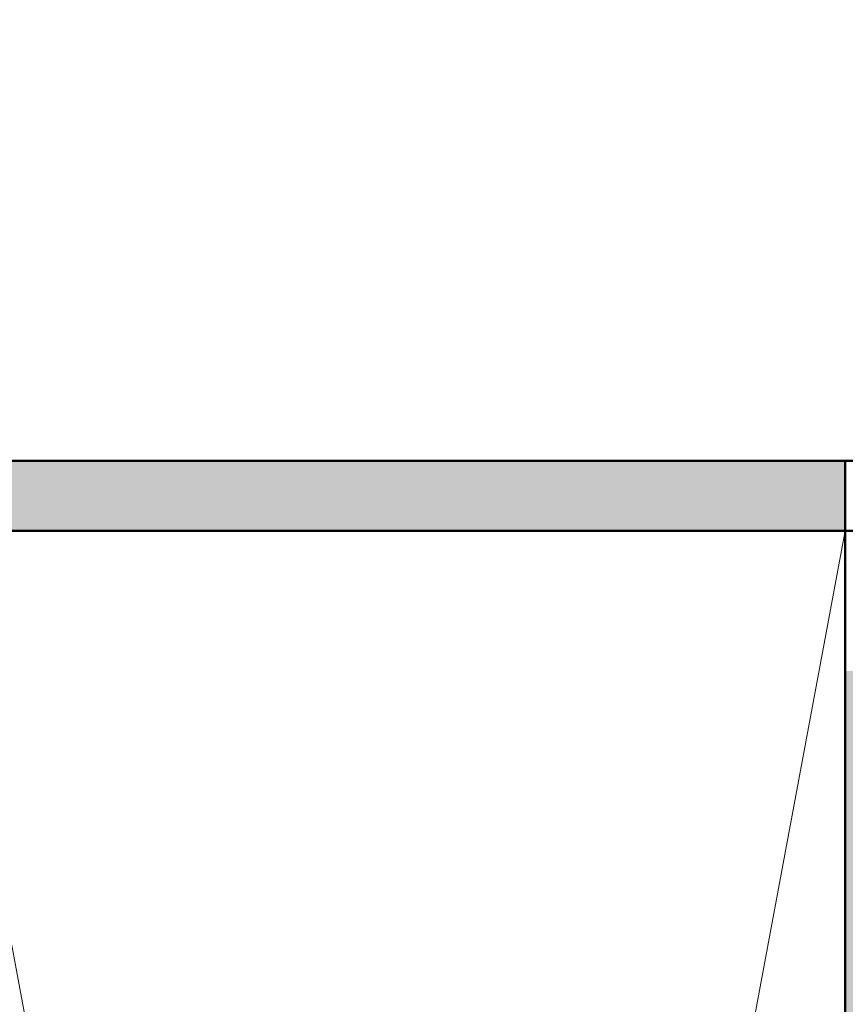
# Model space of a CAD drawing. Units: inches. Extents: x -7 to 1228, y -146 to 1091.
# Tile 28 of 88: x 563 to 634, y 446 to 531. Entities that reach past the tile are written whole.
import ezdxf

# ---------------------------------------------------------------- set-up
doc = ezdxf.new("R2010")
doc.units = ezdxf.units.IN
for name, color, linetype, lineweight in [('A-FLOR-VOID', 7, 'Continuous', 18), ('A-WALL', 7, 'Continuous', 50), ('A-WALL-PATT', 251, 'Continuous', 13)]:
    doc.layers.add(name, color=color, linetype=linetype, lineweight=lineweight)

msp = doc.modelspace()

# ---------------------------------------------------------------- hatches: boundary and pattern name
at = {"layer": 'A-WALL-PATT'}
h = msp.add_hatch(color=256, dxfattribs=at)
h.dxf.hatch_style = 1
h.paths.add_polyline_path([(69, 568), (60, 568), (60, 493), (63.289, 493), (69, 493)])
h.paths.add_polyline_path([(69, 662.405), (60, 662.405), (60, 586), (69, 586)], flags=17)
h.paths.add_polyline_path([(69, 723), (184, 723), (184, 734), (179, 734), (179, 728), (69, 728), (69, 741.623), (60, 741.623), (60, 698.405), (69, 698.405)], flags=17)
h.paths.add_polyline_path([(69, 782), (231, 782), (231, 728), (231, 723), (231, 586), (236, 586), (236, 787), (69, 787), (69, 800.126), (60, 800.126), (60, 765.623), (69, 765.623)])
h.paths.add_polyline_path([(184, 842), (189, 842), (189, 848), (173, 848), (173, 842), (179, 842), (179, 787), (184, 787)])
h.paths.add_polyline_path([(118.22, 69), (69, 69), (69, 60), (118.22, 60)])
h.paths.add_polyline_path([(227, 69), (154.22, 69), (154.22, 60), (227, 60)])
h.paths.add_polyline_path([(236, 60), (232.711, 60), (227, 60), (227, 36), (236, 36)])
h.paths.add_polyline_path([(389, 60), (380, 60), (380, 36), (389, 36)])
h.paths.add_polyline_path([(384, 181), (380, 181), (380, 115), (380, 78), (384, 78)])
h.paths.add_polyline_path([(380, 115), (334.547, 115), (334.547, 109), (380, 109)])
h.paths.add_polyline_path([(274.547, 115), (236, 115), (236, 201), (232.711, 201), (231, 201), (231, 78), (236, 78), (236, 109), (274.547, 109)])
h.paths.add_polyline_path([(69, 123), (60, 123), (60, 78), (69, 78)])
h.paths.add_polyline_path([(69, 201), (60, 201), (60, 159), (69, 159)])
h.paths.add_polyline_path([(143, 219), (69, 219), (69, 213), (143, 213)], flags=17)
h.paths.add_polyline_path([(189, 219), (184, 219), (184, 274), (231, 274), (231, 219), (236, 219), (236, 279), (184, 279), (184, 297), (179, 297), (179, 279), (69, 279), (69, 290.912), (60, 290.912), (60, 262.179), (69, 262.179), (69, 274), (179, 274), (179, 219), (173, 219), (173, 213), (189, 213)])
h.paths.add_polyline_path([(69, 238.179), (60, 238.179), (60, 219), (69, 219)], flags=17)
h.paths.add_polyline_path([(69, 333), (60, 333), (60, 314.912), (69, 314.912), (69, 316.965)])
h.paths.add_polyline_path([(190, 338), (184, 338), (69, 338), (69, 333), (179, 333), (179, 327), (184, 327), (184, 333.021), (190, 333.046)])
h.paths.add_polyline_path([(69, 386.806), (60, 386.806), (60, 351), (69, 351)])
h.paths.add_polyline_path([(69, 475), (60, 475), (60, 422.806), (69, 422.806)])
h.paths.add_polyline_path([(236, 475), (231, 475), (231, 351.238), (236, 351.238)])
h.paths.add_polyline_path([(384, 475), (380, 475), (380, 362), (384, 362)])
h.paths.add_polyline_path([(547, 307), (439, 307), (439, 356), (445, 356), (445, 362), (433, 362), (433, 307), (380, 307), (380, 244), (380, 241), (384, 241), (384, 301), (433, 301), (433, 277), (439, 277), (439, 301), (547, 301)])
h.paths.add_polyline_path([(547, 241), (439, 241), (439, 247), (433, 247), (433, 235), (547, 235)])
h.paths.add_polyline_path([(450, 69), (440.286, 69), (424.889, 69), (389, 69), (389, 60), (450, 60)])
h.paths.add_polyline_path([(547, 69), (486, 69), (486, 60), (547, 60)])
h.paths.add_polyline_path([(556, 148.268), (547, 148.268), (547, 78), (556, 78)])
h.paths.add_polyline_path([(556, 223), (547, 223), (547, 195), (547, 184.268), (556, 184.268)])
h.paths.add_polyline_path([(556, 311.192), (547, 311.192), (547, 273.075), (556, 273.075)])
h.paths.add_polyline_path([(556, 344), (552.711, 344), (547, 344), (547, 335.192), (556, 335.192)])
h.paths.add_polyline_path([(556, 249.075), (547, 249.075), (547, 241), (556, 241)])
h.paths.add_polyline_path([(547, 362), (475, 362), (475, 356), (547, 356)], flags=0)
h.paths.add_polyline_path([(556, 399.621), (547, 399.621), (547, 362), (556, 362)])
h.paths.add_polyline_path([(556, 475), (547, 475), (547, 435.621), (556, 435.621)])
h.paths.add_polyline_path([(547, 493), (389, 493), (389, 487), (547, 487)])
h.paths.add_polyline_path([(380, 493), (278, 493), (278, 487), (380, 487)])
h.paths.add_polyline_path([(227, 493), (69, 493), (69, 487), (227, 487)])
h.paths.add_polyline_path([(643, 122.445), (634, 122.445), (634, 78), (643, 78)])
h.paths.add_polyline_path([(702.5, 69), (692.786, 69), (677.389, 69), (643, 69), (643, 60), (702.5, 60)])
h.paths.add_polyline_path([(798, 69), (738.5, 69), (738.5, 60), (798, 60)])
h.paths.add_polyline_path([(807, 60), (803.711, 60), (798, 60), (798, 36), (807, 36)])
h.paths.add_polyline_path([(807, 109), (846.751, 109), (846.751, 115), (807, 115), (807, 159), (802, 159), (802, 78), (807, 78)])
h.paths.add_polyline_path([(807, 201), (802, 201), (802, 195), (807, 195)])
h.paths.add_polyline_path([(643, 201), (634, 201), (634, 158.445), (643, 158.445)])
h.paths.add_polyline_path([(756, 225), (751, 225), (751, 219), (643, 219), (643, 213), (756, 213)])
h.paths.add_polyline_path([(643, 240.848), (634, 240.848), (634, 219), (643, 219)])
h.paths.add_polyline_path([(643, 274), (643, 288.629), (634, 288.629), (634, 264.848), (643, 264.848)])
h.paths.add_polyline_path([(802, 279), (756, 279), (756, 297), (751, 297), (751, 279), (643, 279), (643, 274), (751, 274), (751, 255), (756, 255), (756, 274), (802, 274)])
h.paths.add_polyline_path([(807, 333), (803.711, 333), (802, 333), (802, 279), (802, 274), (802, 219), (807, 219)])
h.paths.add_polyline_path([(956, 182), (951, 182), (951, 115), (906.751, 115), (906.751, 109), (951, 109), (951, 78), (956, 78)])
h.paths.add_polyline_path([(960, 60), (951, 60), (951, 36), (960, 36)])
h.paths.add_polyline_path([(1021, 69), (1005.781, 69), (960, 69), (960, 60), (1021, 60)])
h.paths.add_polyline_path([(956, 224), (951, 224), (951, 218), (956, 218)])
h.paths.add_polyline_path([(956, 302), (1004, 302), (1004, 278), (1010, 278), (1010, 302), (1118, 302), (1118, 290.809), (1127, 290.809), (1127, 326.968), (1118, 326.968), (1118, 320.966), (1118, 307), (1010, 307), (1010, 356), (1016, 356), (1016, 362), (1004, 362), (1004, 307), (951, 307), (951, 244), (951, 242), (954.289, 242), (956, 242)])
h.paths.add_polyline_path([(643, 333), (634, 333), (634, 312.629), (643, 312.629), (643, 316.965)])
h.paths.add_polyline_path([(756, 338), (643, 338), (643, 333), (751, 333), (751, 327), (756, 327)])
h.paths.add_polyline_path([(643, 388), (634, 388), (634, 351), (643, 351)])
h.paths.add_polyline_path([(807, 357), (802, 357), (802, 351), (807, 351)])
h.paths.add_polyline_path([(807, 475), (802, 475), (802, 393), (807, 393)])
h.paths.add_polyline_path([(643, 475), (634, 475), (634, 424), (643, 424)])
h.paths.add_polyline_path([(798, 493), (643, 493), (643, 487), (798, 487)])
h.paths.add_polyline_path([(634, 493), (556, 493), (556, 487), (634, 487)])
h.paths.add_polyline_path([(813, 493), (807, 493), (807, 487), (813, 487)])
h.paths.add_polyline_path([(951, 493), (849, 493), (849, 487), (951, 487)])
h.paths.add_polyline_path([(956, 484), (951, 484), (951, 374), (956, 374)])
h.paths.add_polyline_path([(1109, 493), (969, 493), (969, 487), (1109, 487)])
h.paths.add_polyline_path([(1127, 484), (1118, 484), (1118, 450.641), (1127, 450.641)])
h.paths.add_polyline_path([(1127, 414.641), (1118, 414.641), (1118, 365), (1127, 365)])
h.paths.add_polyline_path([(1109, 362), (1046, 362), (1046, 356), (1109, 356)], flags=17)
h.paths.add_polyline_path([(1127, 356), (1123.454, 356), (1118, 356), (1118, 350.968), (1127, 350.968)], flags=0)
h.paths.add_polyline_path([(1127, 266.809), (1118, 266.809), (1118, 262.361), (1118, 242), (1127, 242)], flags=17)
h.paths.add_polyline_path([(1118, 242), (1010, 242), (1010, 248), (1004, 248), (1004, 237), (1118, 237)])
h.paths.add_polyline_path([(1127, 224), (1118, 224), (1118, 170), (1127, 170)])
h.paths.add_polyline_path([(1127, 134), (1118, 134), (1118, 78), (1127, 78)])
h.paths.add_polyline_path([(1118, 69), (1057, 69), (1057, 60), (1118, 60)])
h.paths.add_polyline_path([(227, 571.546), (227, 574), (69, 574), (69, 568), (227, 568)])
h.paths.add_polyline_path([(380, 571.546), (380, 574), (278, 574), (278, 568), (380, 568)])
h.paths.add_polyline_path([(242, 574), (236, 574), (236, 568), (242, 568)])
h.paths.add_polyline_path([(547, 571.546), (547, 574), (389, 574), (389, 568), (547, 568)])
h.paths.add_polyline_path([(384, 733), (380, 733), (380, 586), (384, 586)])
h.paths.add_polyline_path([(556, 646), (634, 646), (634, 655), (547, 655), (547, 586), (556, 586)])
h.paths.add_polyline_path([(634, 574), (556, 574), (556, 568), (634, 568)])
h.paths.add_polyline_path([(643, 655), (634, 655), (634, 586), (643, 586)])
h.paths.add_polyline_path([(798, 574), (643, 574), (643, 568), (798, 568)])
h.paths.add_polyline_path([(643, 663.854), (634, 663.854), (634, 655), (643, 655)])
h.paths.add_polyline_path([(556, 676.967), (547, 676.967), (547, 655), (556, 655)])
h.paths.add_polyline_path([(556, 733), (547, 733), (547, 712.967), (556, 712.967)])
h.paths.add_polyline_path([(643, 710), (634, 710), (634, 699.854), (643, 699.854)])
h.paths.add_polyline_path([(807, 668), (802, 668), (802, 586), (807, 586)])
h.paths.add_polyline_path([(951, 574), (849, 574), (849, 568), (951, 568)])
h.paths.add_polyline_path([(956, 691), (951, 691), (951, 577), (956, 577)])
h.paths.add_polyline_path([(1109, 574), (969, 574), (969, 568), (1109, 568)])
h.paths.add_polyline_path([(1127, 643.403), (1118, 643.403), (1118, 577), (1127, 577)])
h.paths.add_polyline_path([(1127, 568), (1123.454, 568), (1118, 568), (1118, 493), (1127, 493)])
h.paths.add_polyline_path([(1127, 733), (1118, 733), (1118, 679.403), (1127, 679.403)])
h.paths.add_polyline_path([(1127, 777.348), (1118, 777.348), (1118, 770.035), (1118, 751), (1127, 751)], flags=17)
h.paths.add_polyline_path([(1118, 751), (1010, 751), (1010, 757), (1004, 757), (1004, 745), (1118, 745)])
h.paths.add_polyline_path([(956, 811), (1004, 811), (1004, 787), (1010, 787), (1010, 811), (1017.874, 811), (1017.874, 811.627, -0.414214), (1018.247, 812), (1031.978, 812, -0.414214), (1032.351, 811.627), (1032.351, 811), (1118, 811), (1118, 801.348), (1127, 801.348), (1127, 834.685), (1118, 834.685), (1118, 830.238), (1118, 817), (1010, 817), (1010, 866), (1016, 866), (1016, 872), (1004, 872), (1004, 817), (956, 817), (956, 866), (951, 866), (951, 751), (954.289, 751), (956, 751)])
h.paths.add_polyline_path([(1118, 872), (1046, 872), (1046, 866), (1118, 866)], flags=17)
h.paths.add_polyline_path([(1127, 924.711), (1118, 924.711), (1118, 884), (1127, 884)])
h.paths.add_polyline_path([(1127, 866), (1123.711, 866), (1118, 866), (1118, 858.685), (1127, 858.685)], flags=17)
h.paths.add_polyline_path([(956, 983), (951, 983), (951, 952), (807, 952), (807, 983), (802, 983), (802, 902), (807, 902), (807, 946), (951, 946), (951, 884), (956, 884)])
h.paths.add_polyline_path([(807, 842), (802, 842), (802, 787), (756, 787), (756, 806), (751, 806), (751, 787), (643, 787), (643, 782), (751, 782), (751, 764), (756, 764), (756, 782), (802, 782), (802, 728), (807, 728)])
h.paths.add_polyline_path([(756, 848), (643, 848), (643, 842), (751, 842), (751, 836), (756, 836)])
h.paths.add_polyline_path([(756, 734), (751, 734), (751, 728), (643, 728), (643, 723), (756, 723)])
h.paths.add_polyline_path([(643, 749.791), (634, 749.791), (634, 728), (637.289, 728), (643, 728)])
h.paths.add_polyline_path([(643, 805.405), (634, 805.405), (634, 773.791), (643, 773.791)])
h.paths.add_polyline_path([(643, 896.663), (634, 896.663), (634, 860), (637.289, 860), (643, 860)])
h.paths.add_polyline_path([(643, 842), (634, 842), (634, 829.405), (643, 829.405)])
h.paths.add_polyline_path([(643, 983), (634, 983), (634, 932.663), (643, 932.663)])
h.paths.add_polyline_path([(1127, 983), (1118, 983), (1118, 960.711), (1127, 960.711)])
h.paths.add_polyline_path([(1118, 1001), (1077.525, 1001), (1077.525, 992), (1118, 992)])
h.paths.add_polyline_path([(1041.525, 1001), (960, 1001), (960, 992), (1041.525, 992)])
h.paths.add_polyline_path([(960, 1025), (951, 1025), (951, 1001), (954.289, 1001), (960, 1001)])
h.paths.add_polyline_path([(807, 1025), (798, 1025), (798, 1001), (807, 1001)])
h.paths.add_polyline_path([(798, 1001), (738.5, 1001), (738.5, 992), (798, 992)])
h.paths.add_polyline_path([(702.5, 1001), (643, 1001), (643, 992), (702.5, 992)])
h.paths.add_polyline_path([(547, 1001), (499.113, 1001), (499.113, 992), (547, 992)])
h.paths.add_polyline_path([(463.113, 1001), (389, 1001), (389, 992), (463.113, 992)])
h.paths.add_polyline_path([(389, 1025), (380, 1025), (380, 1022), (380, 1001), (383.289, 1001), (389, 1001)])
h.paths.add_polyline_path([(236, 1025), (227, 1025), (227, 1001), (236, 1001)])
h.paths.add_polyline_path([(236, 983), (231, 983), (231, 860), (236, 860)])
h.paths.add_polyline_path([(274.547, 952), (236, 952), (236, 946), (274.547, 946)])
h.paths.add_polyline_path([(380, 952), (334.547, 952), (334.547, 946), (380, 946)])
h.paths.add_polyline_path([(384, 983), (380, 983), (380, 884), (383.289, 884), (384, 884)])
h.paths.add_polyline_path([(227, 1001), (155.012, 1001), (155.012, 992), (162.875, 992), (227, 992)])
h.paths.add_polyline_path([(119.012, 1001), (69, 1001), (69, 992), (119.012, 992)])
h.paths.add_polyline_path([(69, 983), (60, 983), (60, 922.987), (69, 922.987)])
h.paths.add_polyline_path([(69, 886.987), (60, 886.987), (60, 860), (63.289, 860), (69, 860)])
h.paths.add_polyline_path([(143, 848), (69, 848), (69, 842), (143, 842)])

# ---------------------------------------------------------------- linework, layer by layer
at = {"layer": 'A-FLOR-VOID'}
for p, q in [((634, 487), (556, 69)), ((556, 487), (634, 69))]:
    msp.add_line(p, q, dxfattribs=at)
at = {"layer": 'A-WALL'}
for p, q in [((813, 493), (556, 493)), ((634, 415), (634, 493)), ((634, 493), (634, 60)), ((813, 487), (556, 487))]:
    msp.add_line(p, q, dxfattribs=at)

doc.saveas('drawing.dxf')
